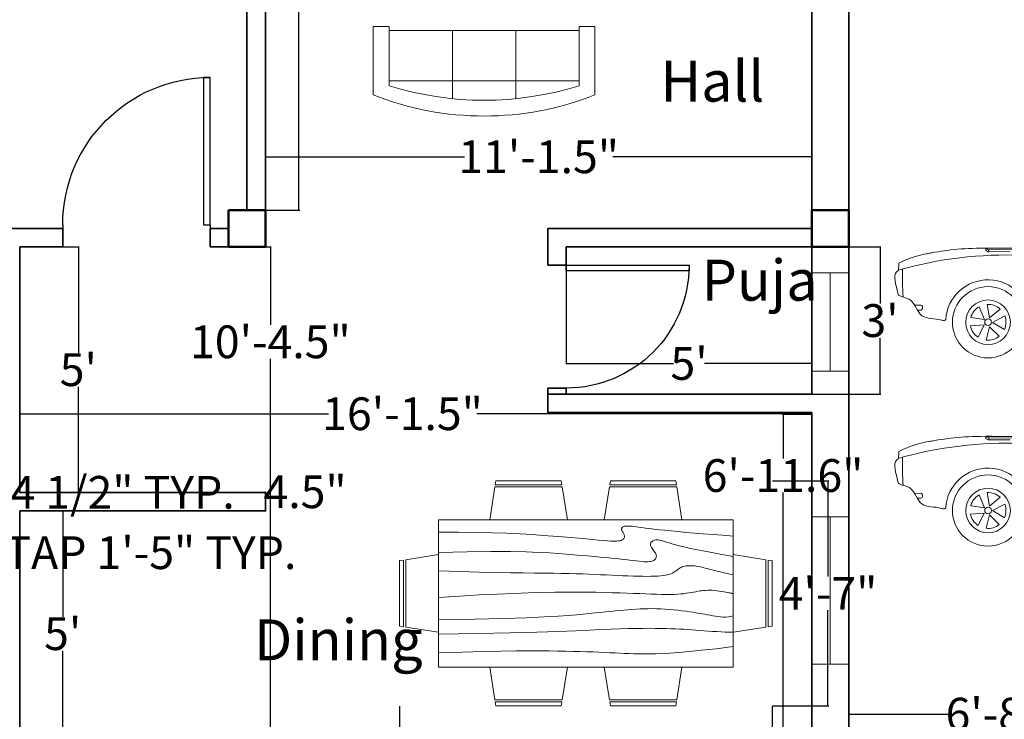
# Model space of a CAD drawing. Units: inches. Extents: x 20414 to 21627, y 49019 to 50314.
# Tile 7 of 10: x 20594 to 20835, y 49988 to 50159. Entities that reach past the tile are written whole.
import ezdxf

# ---------------------------------------------------------------- set-up
doc = ezdxf.new("R2010")
doc.units = ezdxf.units.IN
for name, color, linetype, lineweight in [('A-ANNO-DIMS', 7, 'Continuous', 18), ('A-AREA-IDEN', 7, 'Continuous', 18), ('cars', 40, 'Continuous', 13), ('columns', 1, 'Continuous', 50), ('doors', 3, 'Continuous', 25), ('furniture', 2, 'Continuous', 18), ('walls', 6, 'Continuous', 35), ('windows', 3, 'Continuous', 18)]:
    doc.layers.add(name, color=color, linetype=linetype, lineweight=lineweight)
doc.styles.get("Standard").update_dxf_attribs({"font": 'arial.ttf'})
doc.dimstyles.get("Standard").update_dxf_attribs({"dimtxt": 8, "dimasz": 0.18, "dimexe": 0.18, "dimexo": 0.0625, "dimgap": 0.09, "dimtad": 0, "dimtih": 1, "dimtoh": 1, "dimdec": 1, "dimzin": 0, "dimdsep": 46, "dimlunit": 3, "dimtxsty": 'Standard', "dimcen": 0.09, "dimadec": 0, "dimazin": 0, "dimtfac": 1, "dimtdec": 1, "dimtofl": 0, "dimtmove": 0, "dimatfit": 3, "dimfxl": 1, "dimtolj": 1, "dimtzin": 0, "dimarcsym": 0})

# ---------------------------------------------------------------- blocks, each defined once
blk = doc.blocks.new('Dining Set - 36 x 72 in.')
for p, q in [((-22, 27.5), (-22.1562, 26.50042)), ((-5.8416, 26.5), (-22.1534, 26.5)), ((-22, 27.5), (-6, 27.5)), ((-5.8437, 26.49966), (-6, 27.5)), ((6, 27.5), (5.8438, 26.50042)), ((22.1584, 26.5), (5.8466, 26.5)), ((6, 27.5), (22, 27.5)), ((22.1563, 26.49966), (22, 27.5)), ((-22.2343, 26.00059), (-23.4847, 17.99762)), ((-22.2304, 26), (-5.7608, 26)), ((-4.5152, 17.99762), (-5.7655, 25.99926)), ((5.7657, 26.00059), (4.5153, 17.99762)), ((5.7696, 26), (22.2392, 26)), ((23.4848, 17.99762), (22.2345, 25.99926)), ((36, 18), (-36, 18)), ((-36, 18), (-36, -18)), ((36, -18), (36, 18)), ((-45.5, 8), (-44.5004, 8.15617)), ((-45.5, 8), (-45.5, -8)), ((-44.5, -8.15843), (-44.5, 8.15338)), ((-44.0006, 8.23428), (-35.9976, 9.48474)), ((-44, 8.23041), (-44, -8.23915)), ((44.0006, 8.23428), (35.9976, 9.48474)), ((44, 8.23041), (44, -8.23915)), ((44.5, -8.15843), (44.5, 8.15338)), ((45.5, 8), (44.5005, 8.15617)), ((45.5, 8), (45.5, -8)), ((-44.4997, -8.15631), (-45.5, -8)), ((-35.9976, -9.48476), (-43.9993, -8.2345)), ((35.9976, -9.48476), (43.9993, -8.2345)), ((44.4997, -8.15631), (45.5, -8)), ((-36, -18), (36, -18)), ((-22.2343, -26.0006), (-23.4847, -17.99762)), ((-4.5152, -17.99762), (-5.7655, -25.99928)), ((5.7657, -26.0006), (4.5153, -17.99762)), ((23.4848, -17.99762), (22.2345, -25.99928)), ((-22.2304, -26), (-5.7608, -26)), ((5.7696, -26), (22.2392, -26)), ((-22, -27.5), (-22.1562, -26.50044)), ((-5.8416, -26.5), (-22.1534, -26.5)), ((-22, -27.5), (-6, -27.5)), ((-5.8437, -26.49967), (-6, -27.5)), ((6, -27.5), (5.8438, -26.50044)), ((22.1584, -26.5), (5.8466, -26.5)), ((6, -27.5), (22, -27.5)), ((22.1563, -26.49967), (22, -27.5))]:
    blk.add_line(p, q)
for points in [[(-36, 15), (-31.1772, 14.97754), (-26.8079, 14.91406), (-22.8538, 14.81543), (-19.276, 14.6875), (-16.0362, 14.53613), (-13.0957, 14.36718), (-10.4159, 14.18652), (-7.9583, 14), (-5.6904, 13.81315), (-3.6035, 13.63021), (-1.6954, 13.45508), (0.0365, 13.29166), (1.5945, 13.14388), (2.9811, 13.01562), (4.1988, 12.9108), (5.25, 12.83333), (6.1393, 12.78613), (6.8802, 12.76823), (7.4883, 12.77767), (7.9792, 12.8125), (8.3685, 12.87077), (8.6719, 12.95052), (8.9049, 13.0498), (9.0833, 13.16666), (9.2205, 13.29899), (9.3216, 13.44401), (9.3895, 13.59879), (9.4271, 13.76041), (9.4373, 13.92594), (9.4232, 14.09245), (9.3875, 14.257), (9.3333, 14.41666), (9.2638, 14.56917), (9.1836, 14.71484), (9.0975, 14.85465), (9.0104, 14.98958), (8.9272, 15.1206), (8.8529, 15.2487), (8.7922, 15.37483), (8.75, 15.5), (8.7305, 15.62467), (8.7344, 15.74739), (8.7617, 15.86621), (8.8125, 15.97916), (8.8867, 16.08431), (8.9844, 16.17968), (9.1055, 16.26334), (9.25, 16.33333), (9.4189, 16.38802), (9.6172, 16.42708), (9.8506, 16.45052), (10.125, 16.45833), (10.4463, 16.45052), (10.8203, 16.42708), (11.2529, 16.38802), (11.75, 16.33333), (12.3184, 16.26318), (12.9694, 16.17838), (13.7151, 16.07991), (14.5677, 15.96875), (15.5395, 15.84586), (16.6426, 15.71224), (17.8893, 15.56884), (19.2917, 15.41666), (20.859, 15.25667), (22.5879, 15.08984), (24.4721, 14.91715), (26.5052, 14.73958), (28.6809, 14.5581), (30.9929, 14.3737), (33.4347, 14.18733), (36, 14)], [(-36, 10), (-28.9766, 10.14274), (-23.1725, 10.20442), (-18.4241, 10.19775), (-14.5677, 10.13541), (-11.4399, 10.03011), (-8.877, 9.89453), (-6.7154, 9.74137), (-4.7917, 9.58333), (-2.9698, 9.43082), (-1.2246, 9.28515), (0.4415, 9.14534), (2.026, 9.01041), (3.5266, 8.87939), (4.9408, 8.7513), (6.266, 8.62516), (7.5, 8.5), (8.6411, 8.37549), (9.6914, 8.2539), (10.6538, 8.13818), (11.5312, 8.03125), (12.3267, 7.93603), (13.043, 7.85547), (13.6831, 7.79248), (14.25, 7.75), (14.7471, 7.7303), (15.1797, 7.73307), (15.5537, 7.75732), (15.875, 7.80208), (16.1494, 7.86637), (16.3828, 7.94922), (16.5811, 8.04964), (16.75, 8.16666), (16.8944, 8.29915), (17.0143, 8.44531), (17.1089, 8.60319), (17.1771, 8.77083), (17.218, 8.94629), (17.2305, 9.1276), (17.2137, 9.31282), (17.1667, 9.5), (17.0895, 9.6875), (16.987, 9.875), (16.8649, 10.0625), (16.7292, 10.25), (16.5856, 10.4375), (16.4401, 10.625), (16.2985, 10.8125), (16.1667, 11), (16.05, 11.18733), (15.9518, 11.3737), (15.8752, 11.5581), (15.8229, 11.73958), (15.798, 11.91715), (15.8034, 12.08984), (15.842, 12.25667), (15.9167, 12.41666), (16.0295, 12.56836), (16.1784, 12.70833), (16.3605, 12.83268), (16.5729, 12.9375), (16.8127, 13.01888), (17.0768, 13.07291), (17.3625, 13.0957), (17.6667, 13.08333), (17.9894, 13.03312), (18.3418, 12.94726), (18.7382, 12.82918), (19.1927, 12.68229), (19.7195, 12.51001), (20.3327, 12.31575), (21.0465, 12.10294), (21.875, 11.875), (22.8357, 11.63354), (23.959, 11.37304), (25.2786, 11.08618), (26.8282, 10.76562), (28.6414, 10.40405), (30.752, 9.99414), (33.1936, 9.52856), (36, 9)], [(-36, 5.5), (-30.7157, 5.3348), (-26.069, 5.20963), (-21.9946, 5.11767), (-18.4271, 5.05208), (-15.3009, 5.00602), (-12.5508, 4.97265), (-10.1112, 4.94515), (-7.9167, 4.91666), (-5.909, 4.88167), (-4.0586, 4.83984), (-2.3429, 4.79215), (-0.7396, 4.73958), (0.7739, 4.6831), (2.22, 4.6237), (3.6213, 4.56233), (5, 4.5), (6.373, 4.43782), (7.7344, 4.3776), (9.0723, 4.32129), (10.375, 4.27083), (11.6309, 4.22819), (12.8281, 4.19531), (13.9551, 4.17415), (15, 4.16666), (15.954, 4.17448), (16.819, 4.19791), (17.6001, 4.23698), (18.3021, 4.29166), (18.9299, 4.36198), (19.4883, 4.44791), (19.9823, 4.54948), (20.4167, 4.66666), (20.7969, 4.79899), (21.1302, 4.94401), (21.4245, 5.09879), (21.6875, 5.26041), (21.9271, 5.42594), (22.1511, 5.59245), (22.3672, 5.757), (22.5834, 5.91666), (22.8065, 6.06868), (23.0404, 6.21093), (23.2879, 6.34147), (23.5521, 6.45833), (23.8358, 6.55957), (24.142, 6.64323), (24.4735, 6.70735), (24.8334, 6.75), (25.2235, 6.76969), (25.642, 6.76692), (26.0858, 6.74267), (26.5521, 6.69791), (27.0379, 6.63362), (27.5404, 6.55078), (28.0565, 6.45036), (28.5834, 6.33333), (29.1242, 6.19987), (29.7071, 6.04687), (30.3661, 5.87044), (31.1354, 5.66666), (32.0493, 5.43164), (33.142, 5.16146), (34.4475, 4.85221), (36, 4.5)], [(-36, -1), (-30.7915, -0.6591), (-26.0195, -0.38216), (-21.6519, -0.16284), (-17.6563, 0.00521), (-14.0005, 0.12833), (-10.6523, 0.21289), (-7.5796, 0.26522), (-4.75, 0.29166), (-2.134, 0.29793), (0.2878, 0.28711), (2.5317, 0.26163), (4.6146, 0.22396), (6.5529, 0.17651), (8.3633, 0.12174), (10.0623, 0.06209), (11.6667, 0), (13.1899, -0.06201), (14.6341, -0.1211), (15.9982, -0.17432), (17.2813, -0.21875), (18.4823, -0.25147), (19.6003, -0.26953), (20.6343, -0.27002), (21.5834, -0.25), (22.4481, -0.20768), (23.2357, -0.14584), (23.9549, -0.06836), (24.6146, 0.02083), (25.2235, 0.11784), (25.7904, 0.21875), (26.3241, 0.31966), (26.8334, 0.41666), (27.3265, 0.50618), (27.8099, 0.58593), (28.2894, 0.65397), (28.7709, 0.70833), (29.2601, 0.74707), (29.763, 0.76823), (30.2855, 0.76985), (30.8334, 0.75), (31.4088, 0.70784), (31.9994, 0.64713), (32.589, 0.57275), (33.1615, 0.48958), (33.7008, 0.4025), (34.1908, 0.3164), (34.6153, 0.23616), (34.9584, 0.16666), (35.2099, 0.11165), (35.3848, 0.07031), (35.504, 0.04069), (35.5886, 0.02083), (35.6594, 0.00879), (35.7377, 0.0026), (35.8442, 0.00032), (36, 0)], [(-36, -6.5), (-27.1843, -6.31267), (-20.084, -6.1263), (-14.469, -5.9419), (-10.1094, -5.76042), (-6.7752, -5.58285), (-4.2363, -5.41016), (-2.2629, -5.24333), (-0.625, -5.08334), (0.8708, -4.93099), (2.2715, -4.78646), (3.5872, -4.64974), (4.8281, -4.52084), (6.0046, -4.39974), (7.127, -4.28646), (8.2053, -4.18099), (9.25, -4.08334), (10.2705, -3.99382), (11.2734, -3.91407), (12.2647, -3.84603), (13.25, -3.79167), (14.2354, -3.75293), (15.2266, -3.73177), (16.2295, -3.73015), (17.25, -3.75), (18.2912, -3.79248), (19.3451, -3.85547), (20.4009, -3.93604), (21.4479, -4.03125), (22.4754, -4.13819), (23.4727, -4.25391), (24.4289, -4.37549), (25.3334, -4.5), (26.1785, -4.62492), (26.9694, -4.74935), (27.7145, -4.87281), (28.4219, -4.99479), (29.1, -5.11483), (29.7572, -5.23242), (30.4016, -5.34709), (31.0417, -5.45834), (31.6837, -5.56437), (32.3262, -5.65821), (32.9658, -5.73153), (33.599, -5.77604), (34.2224, -5.78345), (34.8327, -5.74545), (35.4264, -5.65373), (36, -5.5)], [(-36, -10), (-26.4022, -9.81299), (-18.4675, -9.62891), (-11.9839, -9.45069), (-6.7396, -9.28125), (-2.5226, -9.12354), (0.8789, -8.98047), (3.6769, -8.85498), (6.0833, -8.75), (8.2767, -8.66765), (10.3021, -8.60677), (12.1712, -8.56543), (13.8958, -8.54167), (15.4876, -8.53353), (16.9583, -8.53907), (18.3197, -8.55632), (19.5834, -8.58334), (20.7616, -8.61841), (21.8685, -8.66081), (22.9188, -8.71004), (23.9271, -8.76563), (24.9081, -8.82707), (25.8763, -8.89388), (26.8465, -8.96558), (27.8334, -9.04167), (28.8474, -9.12118), (29.8828, -9.20117), (30.93, -9.27824), (31.9792, -9.34896), (33.0205, -9.40991), (34.0443, -9.45768), (35.0407, -9.48885), (36, -9.5)], [(-36, -14.5), (-30.0881, -14.33513), (-25.0332, -14.21224), (-20.7312, -14.12647), (-17.0781, -14.07292), (-13.97, -14.04671), (-11.3027, -14.04297), (-8.9724, -14.05681), (-6.875, -14.08334), (-4.9224, -14.11833), (-3.0905, -14.16016), (-1.3709, -14.20785), (0.2448, -14.26042), (1.7647, -14.3169), (3.1973, -14.3763), (4.5507, -14.43767), (5.8333, -14.5), (7.0554, -14.5621), (8.235, -14.62175), (9.3922, -14.67652), (10.5469, -14.72396), (11.7192, -14.76164), (12.929, -14.78711), (14.1965, -14.79794), (15.5417, -14.79167), (16.9933, -14.76424), (18.6152, -14.70508), (20.4804, -14.60197), (22.6615, -14.44271), (25.2312, -14.21509), (28.2624, -13.9069), (31.8277, -13.50594), (36, -13)]]:
    blk.add_lwpolyline(points)
blk = doc.blocks.new('*U13')
for p, q in [((0, 0), (0, -6)), ((40, 0), (40, -6))]:
    blk.add_line(p, q)
blk.add_lwpolyline([(0, 0), (0, 40), (1.75, 40), (1.75, 0)], close=True)
blk.add_arc((0, 0), 40, 0, 90)
blk = doc.blocks.new('*U16')
for p, q in [((0, 0), (0, 6)), ((40, 0), (40, 6))]:
    blk.add_line(p, q)
blk.add_lwpolyline([(0, 0), (0, -40), (1.75, -40), (1.75, 0)], close=True)
blk.add_arc((0, 0), 40, 270, 0)
blk = doc.blocks.new('Sofa - Roundback 7 ft.')
for p, q in [((-12.00002, -32.4421), (-12.00003, -6.5971)), ((11.99997, -32.4421), (11.99998, -6.5971)), ((-36.000027, -34), (-36.000027, -11.4696)), ((-35.999844, -13.3819), (35.9998, -13.3819)), ((35.99998, -34), (35.99998, -11.4696)), ((-36.000027, -32.4421), (35.99998, -32.4421))]:
    blk.add_line(p, q)
for points in [[(-36.000027, -34), (-42.000027, -34), (-42.000027, -8)], [(41.99998, -8), (41.99998, -34), (35.99998, -34)]]:
    blk.add_lwpolyline(points)
for centre, radius, start, end in [((0, -114.25), 114.25, 68.43141, 111.5686), ((-0.00001, -127.1968), 121.1968, 72.72033, 107.2797)]:
    blk.add_arc(centre, radius, start, end)
blk = doc.blocks.new('*U25')
for p, q in [((1852.4, 1021.9), (2179.3, 1350.6)), ((1905, 986), (2237.3, 1320.1)), ((3032.4, 1318.4), (2995.2, 973.3)), ((1273.2, 1043), (871.5, 1041)), ((896.7, 1027.6), (1273.4, 1031.7)), ((1098.9, 1012.1), (892.9, 1010.3)), ((2821.7, 882.2), (3009.4, 879.9)), ((1184.9, 681.5), (3461.8, 679.9)), ((4581.3, 664.7), (4762.8, 670.8)), ((4554.2, 618.6), (4578.4, 571.2)), ((4741.6, 563), (4788.2, 618.9)), ((189.2, 502.4), (247.5, 503)), ((263.5, 487.3), (263.6, 471.4)), ((4638.6, 536.9), (4696.8, 540.4)), ((248, 455.4), (216.8, 455.1)), ((1292.2, 343.5), (1293, 267.3))]:
    blk.add_line(p, q)
for points in [[(896.8, 1014.3), (896.7, 1023, 0.269532), (892.6, 1029.8), (873.3, 1040.5, 0.575383), (867.4, 1037), (867.5, 1028.3, 0.269532), (871.6, 1021.5), (890.9, 1010.8, 0.575383)], [(723.7, 383.5), (853.7, 365.9), (804, 487.2, 0.199906)], [(879.8, 509.4), (903.2, 380.3), (1003.2, 465.1, 0.199906)], [(3628.3, 383.5), (3758.3, 365.9), (3708.6, 487.2, 0.199906)], [(3784.4, 509.4), (3807.8, 380.3), (3907.8, 465.1, 0.199906)], [(1047.7, 399.8), (932.2, 337.7), (1043.8, 268.7, 0.199906)], [(3952.3, 399.8), (3836.8, 337.7), (3948.4, 268.7, 0.199906)], [(795.2, 196.2), (852.1, 314.3), (721.3, 304.5, 0.199906)], [(995.4, 206.3), (900.7, 296.9), (869.6, 169.5, 0.199906)], [(3699.8, 196.2), (3756.7, 314.3), (3625.9, 304.5, 0.199906)], [(3900, 206.3), (3805.3, 296.9), (3774.2, 169.5, 0.199906)]]:
    blk.add_lwpolyline(points, format="xyb", close=True)
for points in [[(4612.2, 697.6), (4610.9, 811.5), (4584.2, 823.7)], [(4612.2, 697.6), (4610.9, 811.5), (4637.3, 824.3)], [(1293, 267.3), (3413.3, 300.4)]]:
    blk.add_lwpolyline(points)
for centre, radius in [((2943.5, 787.5), 15.7), ((888.4, 339), 339), ((3793, 339), 339), ((888.4, 339), 212.1), ((3793, 339), 212.1), ((888.4, 339), 31.7), ((3793, 339), 31.7)]:
    blk.add_circle(centre, radius)
for centre, radius, start, end in [((2910.9, 2669.2), 1507.9, 237.61027, 240.97846), ((2627.7, -2413), 3753.5, 83.81633, 95.97054), ((2425.8, 99.3), 1361.7, 43.27479, 63.56652), ((1861.5, 1282.4), 260.6, 230.42401, 268.00854), ((3687.4, -2156.1), 3200.2, 71.52833, 102.12419), ((1071.4, -2828.2), 3807.8, 87.83928, 105.80965), ((521.5, -80), 1093.6, 98.53035, 116.11198), ((2034.5, -34648.8), 35635.1, 88.42296, 91.3179), ((3005.1, 571.8), 1299.3, 161.43071, 193.23633), ((651.7, 633.6), 2387.7, 351.8279, 8.16738), ((2010.7, 764.8), 1938, 177.57734, 185.52052), ((1159.2, 681.5), 2000.5, 0.85201, 4.65562), ((1204.8, 682), 2000.5, 0.85201, 4.65562), ((1250.4, 682.5), 2000.5, 0.85201, 4.65562), ((4681.3, 819.2), 63.3, 357.93203, 71.52833), ((3812.4, 364.7), 404.3, 49.2263, 189.1528), ((5493, 959), 918.8, 188.46832, 196.53145), ((3725.8, 939.4), 918.8, 344.74319, 352.80633), ((2960.5, 881.4), 1785.2, 353.19423, 357.93203), ((888.4, 339), 403.8, 0.63732, 176.34123), ((3794.8, 420.2), 377, 352.72855, 41.66131), ((4582.4, 633), 31.7, 91.93898, 207.10902), ((4763.9, 639.2), 31.7, 320.16835, 91.93898), ((1159.2, 681.5), 2000.5, 355.26443, 358.86328), ((1204.8, 682), 2000.5, 355.26443, 358.86328), ((1250.4, 682.5), 2000.5, 355.26443, 358.86328), ((4634.8, 600.1), 63.3, 207.10902, 273.46767), ((4693, 603.6), 63.3, 273.46767, 320.16835), ((247.6, 487.2), 15.8, 0.63732, 90.63732), ((247.8, 471.2), 15.8, 270.63732, 0.63732), ((2901.9, 940.5), 1785.2, 344.3985, 346.93849), ((4126.8, 1798.9), 1427, 271.6865, 290.2774)]:
    blk.add_arc(centre, radius, start, end)
blk.add_ellipse((2969, 853.3), major_axis=(-16, -0.2), ratio=0.610043)
for points, knots in [([(289.3, 988.6), (458.8, 1020.9), (785.1, 1067), (1645.1, 1018.9), (1784.3, 1140.8), (2091.8, 1431.9), (2519.3, 1455.4), (2948, 1431.3), (3379.3, 1419.1), (3689.2, 1266.6), (3901.9, 1112.6), (4093.7, 1033.2), (4189, 1009.1), (4249.1, 994.5)], [18.629823, 18.629823, 18.629823, 18.629823, 19.527405, 20.700571, 21.107983, 21.608568, 21.92336, 23.151359, 23.716171, 23.908743, 24.77794, 24.943072, 25.187755, 25.187755, 25.187755, 25.187755]), ([(485.4, 364.8), (482.3, 360.9), (469.9, 350.9), (389.9, 380.9), (233.5, 354), (184.4, 564.4), (76.5, 575.4), (33.6, 599.7), (16.3, 683.7), (-24.4, 799.9), (39.1, 829), (38, 865.2), (37.8, 883.8), (37.8, 890.5), (38.6, 896.5), (40.2, 902)], [16.815853, 16.815853, 16.815853, 16.815853, 16.838212, 16.885395, 17.18439, 17.479846, 17.654423, 17.670693, 17.696923, 18.016358, 18.052739, 18.140805, 18.140805, 18.140805, 18.172382, 18.172382, 18.172382, 18.172382])]:
    blk.add_open_spline(points, degree=3, knots=knots)
blk = doc.blocks.new('*D32')
at = {"layer": 'A-ANNO-DIMS', "color": 0, "lineweight": -2, "transparency": 16777216}
for p, q in [((20654.49, 50125.09), (20654.49, 50125.21)), ((20654.67, 50125.03), (20703.13, 50125.03)), ((20787.81, 50125.03), (20739.36, 50125.03)), ((20787.99, 50125.09), (20787.99, 50125.21))]:
    blk.add_line(p, q, dxfattribs=at)
at = {"layer": 'A-ANNO-DIMS', "color": 0, "transparency": 16777216}
for points in [[(20654.67, 50125.06), (20654.67, 50125), (20654.49, 50125.03)], [(20787.81, 50125.06), (20787.81, 50125), (20787.99, 50125.03)]]:
    blk.add_solid(points, dxfattribs=at)
at = {"layer": 'Defpoints', "color": 0, "transparency": 16777216}
for p in [(20654.49, 50125.03), (20787.99, 50125.03), (20787.99, 50125.03)]:
    blk.add_point(p, dxfattribs=at)
at = {"layer": 'A-ANNO-DIMS', "color": 0, "transparency": 16777216, "insert": (20721.24, 50125.03), "char_height": 8, "attachment_point": 5}
blk.add_mtext('\\A1;11\'-1.5"', dxfattribs=at)
blk = doc.blocks.new('*D33')
at = {"layer": 'A-ANNO-DIMS', "color": 0, "lineweight": -2, "transparency": 16777216}
for p, q in [((20788.05, 50103.01), (20804.81, 50103.01)), ((20804.63, 50102.83), (20804.63, 50089.18)), ((20804.63, 50067.19), (20804.63, 50080.83)), ((20788.05, 50067.01), (20804.81, 50067.01))]:
    blk.add_line(p, q, dxfattribs=at)
at = {"layer": 'A-ANNO-DIMS', "color": 0, "transparency": 16777216}
for points in [[(20804.6, 50102.83), (20804.66, 50102.83), (20804.63, 50103.01)], [(20804.6, 50067.19), (20804.66, 50067.19), (20804.63, 50067.01)]]:
    blk.add_solid(points, dxfattribs=at)
at = {"layer": 'Defpoints', "color": 0, "transparency": 16777216}
for p in [(20787.99, 50103.01), (20804.63, 50103.01), (20787.99, 50067.01)]:
    blk.add_point(p, dxfattribs=at)
at = {"layer": 'A-ANNO-DIMS', "color": 0, "transparency": 16777216, "insert": (20804.63, 50085.01), "char_height": 8, "attachment_point": 5}
blk.add_mtext("\\A1;3'", dxfattribs=at)
blk = doc.blocks.new('*D34')
at = {"layer": 'A-ANNO-DIMS', "color": 0, "lineweight": -2, "transparency": 16777216}
for p, q in [((20727.99, 50102.94), (20727.99, 50074.35)), ((20787.99, 50102.94), (20787.99, 50074.35)), ((20728.17, 50074.53), (20754.22, 50074.53)), ((20787.81, 50074.53), (20761.76, 50074.53))]:
    blk.add_line(p, q, dxfattribs=at)
at = {"layer": 'A-ANNO-DIMS', "color": 0, "transparency": 16777216}
for points in [[(20728.17, 50074.56), (20728.17, 50074.5), (20727.99, 50074.53)], [(20787.81, 50074.56), (20787.81, 50074.5), (20787.99, 50074.53)]]:
    blk.add_solid(points, dxfattribs=at)
at = {"layer": 'Defpoints', "color": 0, "transparency": 16777216}
for p in [(20727.99, 50103.01), (20787.99, 50103.01), (20727.99, 50074.53)]:
    blk.add_point(p, dxfattribs=at)
at = {"layer": 'A-ANNO-DIMS', "color": 0, "transparency": 16777216, "insert": (20757.99, 50074.53), "char_height": 8, "attachment_point": 5}
blk.add_mtext("\\A1;5'", dxfattribs=at)
blk = doc.blocks.new('*D38')
at = {"layer": 'A-ANNO-DIMS', "color": 0, "lineweight": -2, "transparency": 16777216}
for p, q in [((20796.99, 49977.07), (20796.99, 49989.02)), ((20797.17, 49988.84), (20821.84, 49988.84)), ((20877.31, 49988.84), (20852.65, 49988.84)), ((20877.49, 49977.07), (20877.49, 49989.02))]:
    blk.add_line(p, q, dxfattribs=at)
at = {"layer": 'A-ANNO-DIMS', "color": 0, "transparency": 16777216}
for points in [[(20797.17, 49988.87), (20797.17, 49988.81), (20796.99, 49988.84)], [(20877.31, 49988.87), (20877.31, 49988.81), (20877.49, 49988.84)]]:
    blk.add_solid(points, dxfattribs=at)
at = {"layer": 'Defpoints', "color": 0, "transparency": 16777216}
for p in [(20877.49, 49988.84), (20796.99, 49977.01), (20877.49, 49977.01)]:
    blk.add_point(p, dxfattribs=at)
at = {"layer": 'A-ANNO-DIMS', "color": 0, "transparency": 16777216, "insert": (20837.24, 49988.84), "char_height": 8, "attachment_point": 5}
blk.add_mtext('\\A1;6\'-8.5"', dxfattribs=at)
blk = doc.blocks.new('*D47')
at = {"layer": 'A-ANNO-DIMS', "color": 0, "lineweight": -2, "transparency": 16777216}
for p, q in [((20594.55, 50103.01), (20608.99, 50103.01)), ((20608.81, 50102.83), (20608.81, 50077.16)), ((20608.81, 50043.19), (20608.81, 50068.85)), ((20594.55, 50043.01), (20608.99, 50043.01))]:
    blk.add_line(p, q, dxfattribs=at)
at = {"layer": 'A-ANNO-DIMS', "color": 0, "transparency": 16777216}
for points in [[(20608.78, 50102.83), (20608.84, 50102.83), (20608.81, 50103.01)], [(20608.78, 50043.19), (20608.84, 50043.19), (20608.81, 50043.01)]]:
    blk.add_solid(points, dxfattribs=at)
at = {"layer": 'Defpoints', "color": 0, "transparency": 16777216}
for p in [(20594.49, 50103.01), (20594.49, 50043.01), (20608.81, 50043.01)]:
    blk.add_point(p, dxfattribs=at)
at = {"layer": 'A-ANNO-DIMS', "color": 0, "transparency": 16777216, "insert": (20608.81, 50073.01), "char_height": 8, "attachment_point": 5}
blk.add_mtext("\\A1;5'", dxfattribs=at)
blk = doc.blocks.new('*D48')
at = {"layer": 'A-ANNO-DIMS', "color": 0, "lineweight": -2, "transparency": 16777216}
for p, q in [((20594.55, 50038.51), (20605.17, 50038.51)), ((20604.99, 50038.33), (20604.99, 50012.66)), ((20604.99, 49978.69), (20604.99, 50004.35)), ((20594.55, 49978.51), (20605.17, 49978.51))]:
    blk.add_line(p, q, dxfattribs=at)
at = {"layer": 'A-ANNO-DIMS', "color": 0, "transparency": 16777216}
for points in [[(20604.96, 50038.33), (20605.02, 50038.33), (20604.99, 50038.51)], [(20604.96, 49978.69), (20605.02, 49978.69), (20604.99, 49978.51)]]:
    blk.add_solid(points, dxfattribs=at)
at = {"layer": 'Defpoints', "color": 0, "transparency": 16777216}
for p in [(20594.49, 50038.51), (20594.49, 49978.51), (20604.99, 49978.51)]:
    blk.add_point(p, dxfattribs=at)
at = {"layer": 'A-ANNO-DIMS', "color": 0, "transparency": 16777216, "insert": (20604.99, 50008.51), "char_height": 8, "attachment_point": 5}
blk.add_mtext("\\A1;5'", dxfattribs=at)
blk = doc.blocks.new('*D49')
at = {"layer": 'A-ANNO-DIMS', "color": 0, "lineweight": -2, "transparency": 16777216}
for p, q in [((20654.49, 50043.01), (20654.49, 50043.19)), ((20654.49, 50043.19), (20654.67, 50043.19)), ((20654.49, 50038.69), (20654.49, 50042.83)), ((20654.55, 50043.01), (20654.67, 50043.01)), ((20654.55, 50038.51), (20654.67, 50038.51))]:
    blk.add_line(p, q, dxfattribs=at)
at = {"layer": 'A-ANNO-DIMS', "color": 0, "transparency": 16777216}
for points in [[(20654.46, 50042.83), (20654.52, 50042.83), (20654.49, 50043.01)], [(20654.46, 50038.69), (20654.52, 50038.69), (20654.49, 50038.51)]]:
    blk.add_solid(points, dxfattribs=at)
at = {"layer": 'Defpoints', "color": 0, "transparency": 16777216}
for p in [(20654.49, 50043.01), (20654.49, 50043.01), (20654.49, 50038.51)]:
    blk.add_point(p, dxfattribs=at)
at = {"layer": 'A-ANNO-DIMS', "color": 0, "transparency": 16777216, "insert": (20664.18, 50043.19), "char_height": 8, "attachment_point": 5}
blk.add_mtext('\\A1;4.5"', dxfattribs=at)
blk = doc.blocks.new('*D51')
at = {"layer": 'A-ANNO-DIMS', "color": 0, "lineweight": -2, "transparency": 16777216}
for p, q in [((20654.55, 50232.01), (20662.87, 50232.01)), ((20662.69, 50231.83), (20662.69, 50176.18)), ((20662.69, 50112.19), (20662.69, 50167.83)), ((20654.55, 50112.01), (20662.87, 50112.01))]:
    blk.add_line(p, q, dxfattribs=at)
at = {"layer": 'A-ANNO-DIMS', "color": 0, "transparency": 16777216}
for points in [[(20662.66, 50231.83), (20662.72, 50231.83), (20662.69, 50232.01)], [(20662.66, 50112.19), (20662.72, 50112.19), (20662.69, 50112.01)]]:
    blk.add_solid(points, dxfattribs=at)
at = {"layer": 'Defpoints', "color": 0, "transparency": 16777216}
for p in [(20654.49, 50232.01), (20654.49, 50112.01), (20662.69, 50112.01)]:
    blk.add_point(p, dxfattribs=at)
at = {"layer": 'A-ANNO-DIMS', "color": 0, "transparency": 16777216, "insert": (20662.69, 50172.01), "char_height": 8, "attachment_point": 5}
blk.add_mtext("\\A1;10'", dxfattribs=at)
blk = doc.blocks.new('*D52')
at = {"layer": 'A-ANNO-DIMS', "color": 0, "lineweight": -2, "transparency": 16777216}
for p, q in [((20654.55, 50103.01), (20655.89, 50103.01)), ((20655.71, 50102.83), (20655.71, 50083.99)), ((20655.71, 49978.69), (20655.71, 50075.64)), ((20654.55, 49978.51), (20655.89, 49978.51))]:
    blk.add_line(p, q, dxfattribs=at)
at = {"layer": 'A-ANNO-DIMS', "color": 0, "transparency": 16777216}
for points in [[(20655.68, 50102.83), (20655.74, 50102.83), (20655.71, 50103.01)], [(20655.68, 49978.69), (20655.74, 49978.69), (20655.71, 49978.51)]]:
    blk.add_solid(points, dxfattribs=at)
at = {"layer": 'Defpoints', "color": 0, "transparency": 16777216}
for p in [(20654.49, 50103.01), (20654.49, 49978.51), (20655.71, 49978.51)]:
    blk.add_point(p, dxfattribs=at)
at = {"layer": 'A-ANNO-DIMS', "color": 0, "transparency": 16777216, "insert": (20655.71, 50079.82), "char_height": 8, "attachment_point": 5}
blk.add_mtext('\\A1;10\'-4.5"', dxfattribs=at)
blk = doc.blocks.new('*D54')
at = {"layer": 'A-ANNO-DIMS', "color": 0, "lineweight": -2, "transparency": 16777216}
for p, q in [((20594.49, 50062.44), (20594.49, 50062.07)), ((20787.99, 50062.44), (20787.99, 50062.07)), ((20594.67, 50062.25), (20669.88, 50062.25)), ((20787.81, 50062.25), (20706.11, 50062.25))]:
    blk.add_line(p, q, dxfattribs=at)
at = {"layer": 'A-ANNO-DIMS', "color": 0, "transparency": 16777216}
for points in [[(20594.67, 50062.28), (20594.67, 50062.22), (20594.49, 50062.25)], [(20787.81, 50062.28), (20787.81, 50062.22), (20787.99, 50062.25)]]:
    blk.add_solid(points, dxfattribs=at)
at = {"layer": 'Defpoints', "color": 0, "transparency": 16777216}
for p in [(20594.49, 50062.51), (20787.99, 50062.51), (20594.49, 50062.25)]:
    blk.add_point(p, dxfattribs=at)
at = {"layer": 'A-ANNO-DIMS', "color": 0, "transparency": 16777216, "insert": (20687.99, 50062.25), "char_height": 8, "attachment_point": 5}
blk.add_mtext('\\A1;16\'-1.5"', dxfattribs=at)
blk = doc.blocks.new('*D58')
at = {"layer": 'A-ANNO-DIMS', "color": 0, "lineweight": -2, "transparency": 16777216}
for p, q in [((20787.93, 50062.07), (20780.76, 50062.07)), ((20780.94, 50061.89), (20780.94, 50051.32)), ((20780.94, 49978.69), (20780.94, 50042.97)), ((20787.93, 49978.51), (20780.76, 49978.51))]:
    blk.add_line(p, q, dxfattribs=at)
at = {"layer": 'A-ANNO-DIMS', "color": 0, "transparency": 16777216}
for points in [[(20780.91, 50061.89), (20780.97, 50061.89), (20780.94, 50062.07)], [(20780.91, 49978.69), (20780.97, 49978.69), (20780.94, 49978.51)]]:
    blk.add_solid(points, dxfattribs=at)
at = {"layer": 'Defpoints', "color": 0, "transparency": 16777216}
for p in [(20780.94, 50062.07), (20787.99, 50062.07), (20787.99, 49978.51)]:
    blk.add_point(p, dxfattribs=at)
at = {"layer": 'A-ANNO-DIMS', "color": 0, "transparency": 16777216, "insert": (20780.94, 50047.15), "char_height": 8, "attachment_point": 5}
blk.add_mtext('\\A1;6\'-11.6"', dxfattribs=at)
blk = doc.blocks.new('WINDOW-36IN-PLAN')
for p, q in [((9, 36), (0, 36)), ((4.5, 36), (4.5, 0)), ((9, 0), (0, 0))]:
    blk.add_line(p, q)
blk = doc.blocks.new('VENT-24IN-PLAN')
for p, q in [((9, 24), (0, 24)), ((4.5, 0), (4.5, 24)), ((9, 0), (0, 0))]:
    blk.add_line(p, q)
blk = doc.blocks.new('COLUMN-9X9')
blk.add_lwpolyline([(0, 9), (0, 0), (9, 0), (9, 9), (0, 9)])
blk = doc.blocks.new('*D93')
at = {"layer": 'A-ANNO-DIMS', "color": 0, "lineweight": -2, "transparency": 16777216}
for p, q in [((20574.69, 50043.81), (20574.71, 50042.8)), ((20579.19, 50043.88), (20579.21, 50042.86)), ((20574.88, 50042.98), (20579.02, 50043.04)), ((20579.2, 50043.04), (20579.38, 50043.04))]:
    blk.add_line(p, q, dxfattribs=at)
at = {"layer": 'A-ANNO-DIMS', "color": 0, "transparency": 16777216}
for points in [[(20574.88, 50043.01), (20574.88, 50042.95), (20574.7, 50042.98)], [(20579.02, 50043.07), (20579.02, 50043.01), (20579.2, 50043.04)]]:
    blk.add_solid(points, dxfattribs=at)
at = {"layer": 'Defpoints', "color": 0, "transparency": 16777216}
for p in [(20574.69, 50043.88), (20579.19, 50043.94), (20579.2, 50043.04)]:
    blk.add_point(p, dxfattribs=at)
at = {"layer": 'A-ANNO-DIMS', "color": 0, "transparency": 16777216, "insert": (20613.18, 50043.04), "char_height": 8, "attachment_point": 5}
blk.add_mtext('\\A1;0\'-4 1/2" TYP.', dxfattribs=at)
blk = doc.blocks.new('*D96')
at = {"layer": 'A-ANNO-DIMS', "color": 0, "lineweight": -2, "transparency": 16777216}
for p, q in [((20540.67, 50030.79), (20540.67, 50028.12)), ((20557.68, 50030.79), (20557.68, 50028.12)), ((20540.85, 50028.3), (20557.5, 50028.3)), ((20557.68, 50028.3), (20557.86, 50028.3))]:
    blk.add_line(p, q, dxfattribs=at)
at = {"layer": 'A-ANNO-DIMS', "color": 0, "transparency": 16777216}
for points in [[(20540.85, 50028.33), (20540.85, 50028.27), (20540.67, 50028.3)], [(20557.5, 50028.33), (20557.5, 50028.27), (20557.68, 50028.3)]]:
    blk.add_solid(points, dxfattribs=at)
at = {"layer": 'Defpoints', "color": 0, "transparency": 16777216}
for p in [(20540.67, 50030.85), (20557.68, 50030.85), (20557.68, 50028.3)]:
    blk.add_point(p, dxfattribs=at)
at = {"layer": 'A-ANNO-DIMS', "color": 0, "transparency": 16777216, "insert": (20611.03, 50028.3), "char_height": 8, "attachment_point": 5}
blk.add_mtext('\\A1;BATH TAP 1\'-5" TYP.', dxfattribs=at)
blk = doc.blocks.new('*D116')
at = {"layer": 'A-ANNO-DIMS', "color": 0, "lineweight": -2, "transparency": 16777216}
for p, q in [((20687.27, 49990.79), (20687.27, 49977.02)), ((20778.27, 49990.79), (20778.27, 49977.02)), ((20687.45, 49977.2), (20688.71, 49977.2)), ((20778.09, 49977.2), (20776.82, 49977.2))]:
    blk.add_line(p, q, dxfattribs=at)
at = {"layer": 'A-ANNO-DIMS', "color": 0, "transparency": 16777216}
for points in [[(20687.45, 49977.23), (20687.45, 49977.17), (20687.27, 49977.2)], [(20778.09, 49977.23), (20778.09, 49977.17), (20778.27, 49977.2)]]:
    blk.add_solid(points, dxfattribs=at)
at = {"layer": 'Defpoints', "color": 0, "transparency": 16777216}
for p in [(20687.27, 49990.85), (20778.27, 49990.85), (20778.27, 49977.2)]:
    blk.add_point(p, dxfattribs=at)
at = {"layer": 'A-ANNO-DIMS', "color": 0, "transparency": 16777216, "insert": (20732.77, 49977.2), "char_height": 8, "attachment_point": 5}
blk.add_mtext('\\A1;DINING SET 7\'-7"', dxfattribs=at)
blk = doc.blocks.new('*D117')
at = {"layer": 'A-ANNO-DIMS', "color": 0, "lineweight": -2, "transparency": 16777216}
for p, q in [((20778.33, 50045.85), (20792.1, 50045.85)), ((20791.92, 50045.67), (20791.92, 50022.44)), ((20791.92, 49991.03), (20791.92, 50014.26)), ((20778.33, 49990.85), (20792.1, 49990.85))]:
    blk.add_line(p, q, dxfattribs=at)
at = {"layer": 'A-ANNO-DIMS', "color": 0, "transparency": 16777216}
for points in [[(20791.89, 50045.67), (20791.95, 50045.67), (20791.92, 50045.85)], [(20791.89, 49991.03), (20791.95, 49991.03), (20791.92, 49990.85)]]:
    blk.add_solid(points, dxfattribs=at)
at = {"layer": 'Defpoints', "color": 0, "transparency": 16777216}
for p in [(20778.27, 50045.85), (20791.92, 50045.85), (20778.27, 49990.85)]:
    blk.add_point(p, dxfattribs=at)
at = {"layer": 'A-ANNO-DIMS', "color": 0, "transparency": 16777216, "insert": (20791.92, 50018.35), "char_height": 8, "attachment_point": 5}
blk.add_mtext('\\A1;4\'-7"', dxfattribs=at)

msp = doc.modelspace()

# ---------------------------------------------------------------- linework, layer by layer
at = {"layer": 'walls'}
for p, q in [((20649.99, 50112.01), (20649.99, 50232.01)), ((20654.49, 50103.01), (20654.49, 50232.01)), ((20787.99, 50172.01), (20787.99, 50107.51)), ((20796.99, 50172.01), (20796.99, 49821.01)), ((20604.99, 50107.51), (20584.86, 50107.51)), ((20604.99, 50103.01), (20604.99, 50107.51)), ((20645.49, 50107.51), (20640.99, 50107.51)), ((20640.99, 50103.01), (20640.99, 50107.51)), ((20787.99, 50107.51), (20723.49, 50107.51)), ((20723.49, 50107.51), (20723.49, 50098.51)), ((20594.49, 50043.01), (20594.49, 50103.01)), ((20604.99, 50103.01), (20594.49, 50103.01)), ((20654.49, 50103.01), (20640.99, 50103.01)), ((20787.99, 50103.01), (20727.99, 50103.01)), ((20727.99, 50103.01), (20727.99, 50098.51)), ((20787.99, 50103.01), (20787.99, 50067.01)), ((20727.99, 50098.51), (20723.49, 50098.51)), ((20727.99, 50068.51), (20723.49, 50068.51)), ((20723.49, 50068.51), (20723.49, 50062.51)), ((20727.99, 50068.51), (20727.99, 50067.01)), ((20727.99, 50067.01), (20723.49, 50067.01)), ((20787.99, 50067.01), (20727.99, 50067.01)), ((20787.99, 50062.51), (20723.49, 50062.51)), ((20787.99, 50062.51), (20787.99, 49978.51)), ((20654.49, 50043.01), (20594.49, 50043.01)), ((20654.49, 50038.51), (20654.49, 50043.01)), ((20654.49, 50038.51), (20594.49, 50038.51)), ((20594.49, 49978.51), (20594.49, 50038.51))]:
    msp.add_line(p, q, dxfattribs=at)

# ---------------------------------------------------------------- block references
at = {"layer": 'cars', "xscale": 0.025666680406073, "yscale": 0.025666680406073, "zscale": 0.025666680406073}
for p in [(20808.22, 50075.9), (20808.22, 50029.9)]:
    msp.add_blockref('*U25', p, dxfattribs=at)
at = {"layer": 'columns'}
for p in [(20645.49, 50103.01), (20787.99, 50103.01)]:
    msp.add_blockref('COLUMN-9X9', p, dxfattribs=at)
at = {"layer": 'doors', "xscale": -0.9, "yscale": 0.9, "zscale": 0.9}
msp.add_blockref('*U13', (20640.99, 50108.41), dxfattribs=at)
at = {"layer": 'doors', "xscale": -0.75, "yscale": 0.75, "zscale": 0.75, "rotation": 90}
msp.add_blockref('*U16', (20727.99, 50098.51), dxfattribs=at)
at = {"layer": 'furniture', "xscale": -0.6442431863649634, "yscale": 0.6442431863649634, "zscale": 0.6442431863649634, "rotation": 180}
msp.add_blockref('Sofa - Roundback 7 ft.', (20707.92, 50134.98), dxfattribs=at)
at = {"layer": 'furniture'}
msp.add_blockref('Dining Set - 36 x 72 in.', (20732.77, 50018.35), dxfattribs=at)
at = {"layer": 'windows'}
msp.add_blockref('VENT-24IN-PLAN', (20787.99, 50072.68), dxfattribs=at)
at = {"layer": 'windows', "rotation": 180}
msp.add_blockref('WINDOW-36IN-PLAN', (20796.99, 50037.03), dxfattribs=at)

# ---------------------------------------------------------------- texts
at = {"layer": 'A-AREA-IDEN', "char_height": 10, "attachment_point": 1}
for s, insert in [('Hall', (20751.01, 50148.51)), ('Puja', (20761.05, 50099.89)), ('Dining', (20651.68, 50012.01))]:
    msp.add_mtext_dynamic_manual_height_columns(s, width=44.4717, gutter_width=50, heights=[34.97], dxfattribs=dict(at, insert=insert))

# ---------------------------------------------------------------- dimensions: what is measured, and where the dimension line sits
at = {"layer": 'A-ANNO-DIMS'}
for base, p1, p2, override, picture, middle in [((20662.69, 50112.01), (20654.49, 50232.01), (20654.49, 50112.01), {"dimclrd": 0, "dimclre": 0, "dimclrt": 0}, '*D51', (20662.69, 50172.01)), ((20608.81, 50043.01), (20594.49, 50103.01), (20594.49, 50043.01), {"dimclrd": 0, "dimclre": 0, "dimclrt": 0}, '*D47', (20608.81, 50073.01)), ((20804.63, 50103.01), (20787.99, 50067.01), (20787.99, 50103.01), {"dimclrd": 0, "dimclre": 0, "dimclrt": 0}, '*D33', (20804.63, 50085.01)), ((20654.49, 50043.01), (20654.49, 50038.51), (20654.49, 50043.01), {"dimclrd": 0, "dimclre": 0, "dimclrt": 0}, '*D49', (20664.18, 50043.19)), ((20791.92, 50045.85), (20778.27, 49990.85), (20778.27, 50045.85), {"dimdec": 1, "dimlfac": 1, "dimrnd": 0, "dimzin": 1, "dimdsep": 46, "dimlunit": 4, "dimfrac": 2}, '*D117', (20791.92, 50018.35)), ((20604.99, 49978.51), (20594.49, 50038.51), (20594.49, 49978.51), {"dimclrd": 0, "dimclre": 0, "dimclrt": 0}, '*D48', (20604.99, 50008.51))]:
    dim = msp.add_linear_dim(base=base, p1=p1, p2=p2, angle=90, dimstyle='Standard', override=override, dxfattribs=at)
    dim.commit()
    dim.dimension.update_dxf_attribs({"geometry": picture, "text_midpoint": middle})
for base, p1, p2, picture, middle in [((20787.99, 50125.03), (20654.49, 50125.03), (20787.99, 50125.03), '*D32', (20721.24, 50125.03)), ((20727.99, 50074.53), (20787.99, 50103.01), (20727.99, 50103.01), '*D34', (20757.99, 50074.53)), ((20877.49, 49988.84), (20796.99, 49977.01), (20877.49, 49977.01), '*D38', (20837.24, 49988.84))]:
    dim = msp.add_linear_dim(base=base, p1=p1, p2=p2, dimstyle='Standard', override={"dimclrd": 0, "dimclre": 0, "dimclrt": 0}, dxfattribs=at)
    dim.commit()
    dim.dimension.update_dxf_attribs({"geometry": picture, "text_midpoint": middle})
for base, p1, p2, picture, middle in [((20655.71, 49978.51), (20654.49, 50103.01), (20654.49, 49978.51), '*D52', (20655.71, 50079.82)), ((20780.94, 50062.07), (20787.99, 49978.51), (20787.99, 50062.07), '*D58', (20780.94, 50047.15))]:
    dim = msp.add_linear_dim(base=base, p1=p1, p2=p2, angle=90, dimstyle='Standard', override={"dimclrd": 0, "dimclre": 0, "dimclrt": 0}, dxfattribs=at)
    dim.commit()
    dim.dimension.update_dxf_attribs({"geometry": picture, "text_midpoint": middle, "dimtype": 160})
dim = msp.add_linear_dim(base=(20594.49, 50062.25), p1=(20787.99, 50062.51), p2=(20594.49, 50062.51), dimstyle='Standard', override={"dimclrd": 0, "dimclre": 0, "dimclrt": 0}, dxfattribs=at)
dim.commit()
dim.dimension.update_dxf_attribs({"geometry": '*D54', "text_midpoint": (20687.99, 50062.25), "dimtype": 160})
dim = msp.add_linear_dim(base=(20579.2, 50043.04), p1=(20574.69, 50043.88), p2=(20579.19, 50043.94), angle=0.8034, text='<> TYP.', dimstyle='Standard', override={"dimdec": 1, "dimlfac": 1, "dimrnd": 0, "dimzin": 1, "dimdsep": 46, "dimlunit": 4, "dimfrac": 2}, dxfattribs=at)
dim.commit()
dim.dimension.update_dxf_attribs({"geometry": '*D93', "text_midpoint": (20613.18, 50043.04)})
for base, p1, p2, text, picture, middle in [((20557.68, 50028.3), (20540.67, 50030.85), (20557.68, 50030.85), 'BATH TAP <> TYP.', '*D96', (20611.03, 50028.3)), ((20778.27, 49977.2), (20687.27, 49990.85), (20778.27, 49990.85), 'DINING SET <>', '*D116', (20732.77, 49977.2))]:
    dim = msp.add_linear_dim(base=base, p1=p1, p2=p2, text=text, dimstyle='Standard', override={"dimdec": 1, "dimlfac": 1, "dimrnd": 0, "dimzin": 1, "dimdsep": 46, "dimlunit": 4, "dimfrac": 2}, dxfattribs=at)
    dim.commit()
    dim.dimension.update_dxf_attribs({"geometry": picture, "text_midpoint": middle})

doc.saveas('drawing.dxf')
